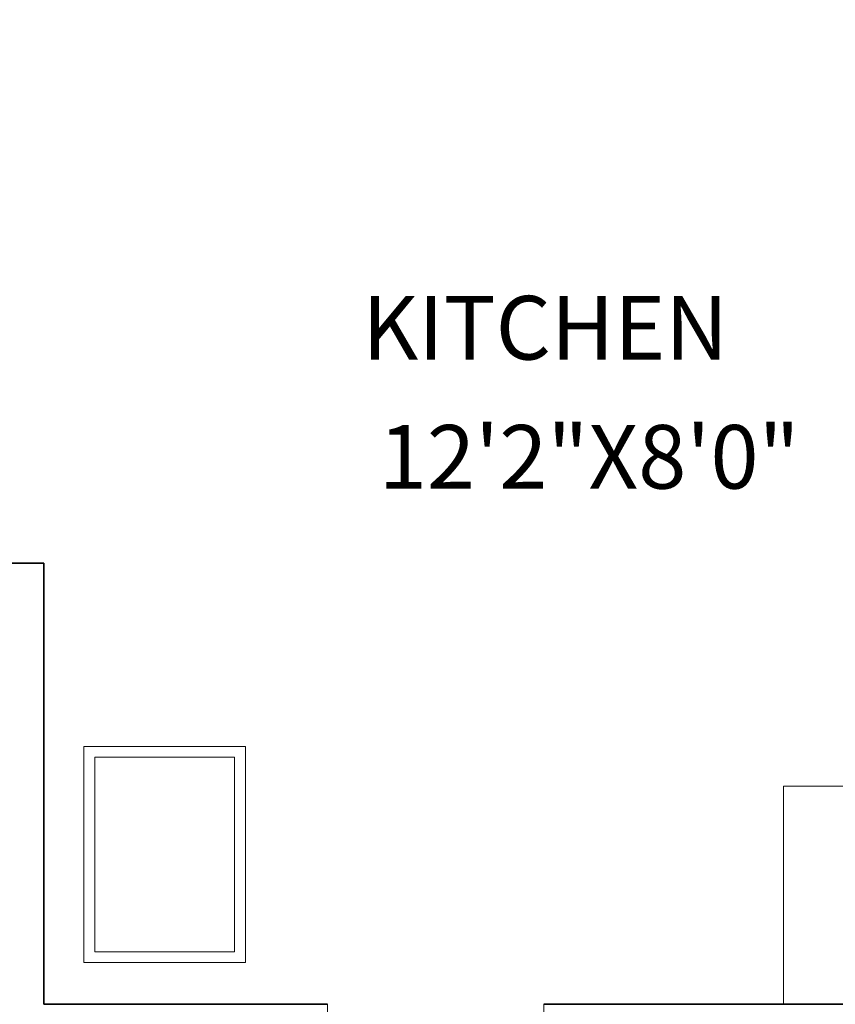
# Model space of a CAD drawing. Units: millimetres. Extents: x 27017497 to 27018854, y 7058029 to 7059154.
# Tile 49 of 91: x 27017886 to 27017962, y 7058203 to 7058294. Entities that reach past the tile are written whole.
import ezdxf

# ---------------------------------------------------------------- set-up
doc = ezdxf.new("R2010")
doc.units = ezdxf.units.MM
for name, color, linetype, lineweight in [('A-ANNO-DIMS', 2, 'Continuous', 18), ('A-AREA-IDEN', 7, 'Continuous', 18), ('A-DOOR', 4, 'Continuous', 20), ('A-EQPM', 9, 'Continuous', 18), ('A-FLOR-CASE', 8, 'Continuous', 20), ('A-WALL', 7, 'Continuous', 35)]:
    doc.layers.add(name, color=color, linetype=linetype, lineweight=lineweight)
doc.styles.get("Standard").update_dxf_attribs({"font": 'arial.ttf'})
doc.dimstyles.get("Standard").update_dxf_attribs({"dimtxt": 0.18, "dimasz": 0.18, "dimexe": 0.18, "dimexo": 0.0625, "dimgap": 0.09, "dimtad": 0, "dimtih": 1, "dimtoh": 1, "dimdec": 4, "dimzin": 0, "dimdsep": 46, "dimtxsty": 'Standard', "dimcen": 0.09, "dimadec": 0, "dimazin": 0, "dimtfac": 1, "dimtdec": 4, "dimtofl": 0, "dimtmove": 0, "dimatfit": 3, "dimfxl": 1, "dimtolj": 1, "dimtzin": 0, "dimarcsym": 0})

# ---------------------------------------------------------------- blocks, each defined once
blk = doc.blocks.new('*U2')
for p, q in [((0, 0), (0, -6)), ((40, 0), (40, -6))]:
    blk.add_line(p, q)
blk.add_lwpolyline([(0, 0), (0, 40), (1.75, 40), (1.75, 0)], close=True)
blk.add_arc((0, 0), 40, 0, 90)
blk = doc.blocks.new('*D47')
at = {"layer": 'A-ANNO-DIMS', "color": 0, "lineweight": -2, "transparency": 16777216}
for p, q in [((27017561.166, 7058294.35), (27017561.166, 7058028.6)), ((27018790.606, 7058294.35), (27018790.606, 7058028.6)), ((27017561.346, 7058028.78), (27018175.431, 7058028.78)), ((27018790.426, 7058028.78), (27018176.341, 7058028.78))]:
    blk.add_line(p, q, dxfattribs=at)
at = {"layer": 'A-ANNO-DIMS', "color": 0, "transparency": 16777216}
for points in [[(27017561.346, 7058028.81), (27017561.346, 7058028.75), (27017561.166, 7058028.78)], [(27018790.426, 7058028.81), (27018790.426, 7058028.75), (27018790.606, 7058028.78)]]:
    blk.add_solid(points, dxfattribs=at)
at = {"layer": 'Defpoints', "color": 0, "transparency": 16777216}
for p in [(27017561.166, 7058294.412), (27018790.606, 7058294.412), (27018790.606, 7058028.78)]:
    blk.add_point(p, dxfattribs=at)
at = {"layer": 'A-ANNO-DIMS', "color": 0, "transparency": 16777216, "insert": (27018175.886, 7058028.78), "char_height": 0.18, "attachment_point": 5}
blk.add_mtext('\\A1;1229.4', dxfattribs=at)
blk = doc.blocks.new('*D48')
at = {"layer": 'A-ANNO-DIMS', "color": 0, "lineweight": -2, "transparency": 16777216}
for p, q in [((27018463.498, 7058622.912), (27017497.536, 7058622.912)), ((27017497.716, 7058622.732), (27017497.716, 7058357.753)), ((27017497.716, 7058092.41), (27017497.716, 7058357.389)), ((27018555.129, 7058092.23), (27017497.536, 7058092.23))]:
    blk.add_line(p, q, dxfattribs=at)
at = {"layer": 'A-ANNO-DIMS', "color": 0, "transparency": 16777216}
for points in [[(27017497.686, 7058622.732), (27017497.746, 7058622.732), (27017497.716, 7058622.912)], [(27017497.686, 7058092.41), (27017497.746, 7058092.41), (27017497.716, 7058092.23)]]:
    blk.add_solid(points, dxfattribs=at)
at = {"layer": 'Defpoints', "color": 0, "transparency": 16777216}
for p in [(27018463.561, 7058622.912), (27017497.716, 7058092.23), (27018555.192, 7058092.23)]:
    blk.add_point(p, dxfattribs=at)
at = {"layer": 'A-ANNO-DIMS', "color": 0, "transparency": 16777216, "insert": (27017497.716, 7058357.571), "char_height": 0.18, "attachment_point": 5}
blk.add_mtext('\\A1;530.7', dxfattribs=at)

msp = doc.modelspace()

# ---------------------------------------------------------------- linework, layer by layer
at = {"layer": 'A-EQPM'}
for p, q in [((27017891.888, 7058226.869), (27017891.888, 7058206.794)), ((27017906.893, 7058226.869), (27017891.888, 7058226.869)), ((27017906.893, 7058206.794), (27017906.893, 7058226.869)), ((27017905.893, 7058225.869), (27017892.888, 7058225.869)), ((27017892.888, 7058225.869), (27017892.888, 7058207.794)), ((27017905.893, 7058207.794), (27017905.893, 7058225.869)), ((27017892.888, 7058207.794), (27017905.893, 7058207.794)), ((27017891.888, 7058206.794), (27017906.893, 7058206.794))]:
    msp.add_line(p, q, dxfattribs=at)
at = {"layer": 'A-FLOR-CASE'}
for p, q in [((27018004.365, 7058223.172), (27017956.932, 7058223.172)), ((27017956.932, 7058223.172), (27017956.932, 7058202.912))]:
    msp.add_line(p, q, dxfattribs=at)
at = {"layer": 'A-WALL'}
for p, q in [((27017806.666, 7058243.912), (27017888.166, 7058243.912)), ((27017888.166, 7058243.912), (27017888.166, 7058202.912)), ((27017888.166, 7058202.912), (27017914.524, 7058202.912)), ((27017934.651, 7058202.912), (27018032.166, 7058202.912))]:
    msp.add_line(p, q, dxfattribs=at)

# ---------------------------------------------------------------- block references
at = {"layer": 'A-DOOR', "xscale": -0.503175151877956, "yscale": 0.503175151877956, "zscale": 0.503175151877956, "rotation": 180}
msp.add_blockref('*U2', (27017914.524, 7058199.894), dxfattribs=at)

# ---------------------------------------------------------------- texts
at = {"layer": 'A-ANNO-DIMS'}
msp.add_text('12\'2"X8\'0"', height=5.9118, dxfattribs=at).set_placement((27017919.298, 7058250.834))
at = {"layer": 'A-AREA-IDEN'}
msp.add_text('KITCHEN', height=5.9118, dxfattribs=at).set_placement((27017917.762, 7058262.831))

# ---------------------------------------------------------------- dimensions: what is measured, and where the dimension line sits
at = {"layer": 'A-ANNO-DIMS'}
dim = msp.add_linear_dim(base=(27017497.716, 7058092.23), p1=(27018463.561, 7058622.912), p2=(27018555.192, 7058092.23), angle=90, dimstyle='Standard', override={"dimdec": 1, "dimlfac": 1, "dimrnd": 0, "dimzin": 0, "dimdsep": 46, "dimlunit": 2}, dxfattribs=at)
dim.commit()
dim.dimension.update_dxf_attribs({"geometry": '*D48', "text_midpoint": (27017497.716, 7058357.571)})
dim = msp.add_linear_dim(base=(27018790.606, 7058028.78), p1=(27017561.166, 7058294.412), p2=(27018790.606, 7058294.412), dimstyle='Standard', override={"dimdec": 1, "dimlfac": 1, "dimrnd": 0, "dimzin": 0, "dimdsep": 46, "dimlunit": 2}, dxfattribs=at)
dim.commit()
dim.dimension.update_dxf_attribs({"geometry": '*D47', "text_midpoint": (27018175.886, 7058028.78)})

doc.saveas('drawing.dxf')
